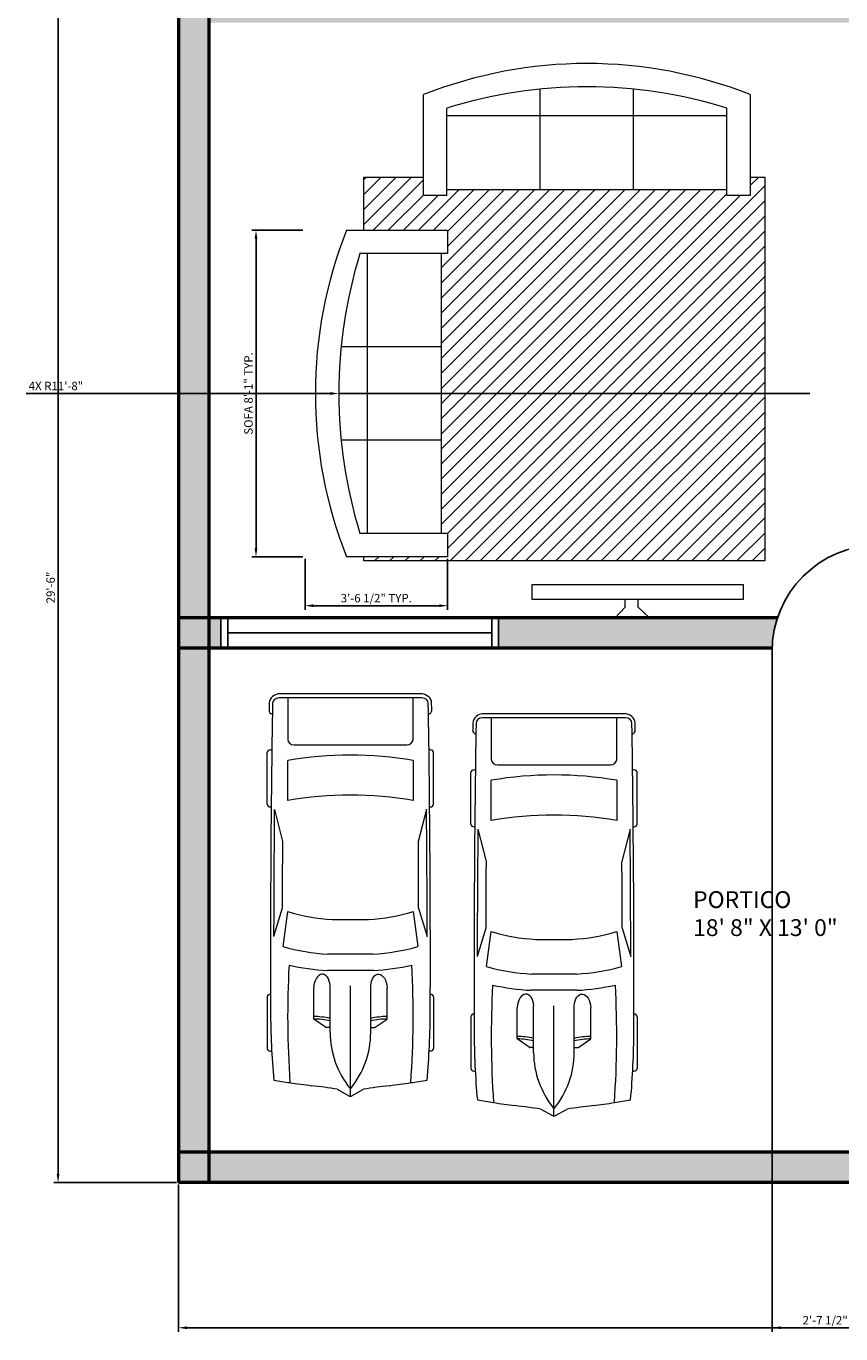
# Model space of a CAD drawing. Units: millimetres. Extents: x 2481 to 3088, y 720 to 1513.
# Tile 1 of 4: x 2481 to 2723, y 720 to 1109. Entities that reach past the tile are written whole.
import ezdxf

# ---------------------------------------------------------------- set-up
doc = ezdxf.new("R2010")
doc.units = ezdxf.units.MM
for name, color, linetype, lineweight in [('A-EQPM', 2, 'Continuous', 18), ('A-SITE-VEHC', 2, 'Continuous', 13), ('A-WALL-PATT', 5, 'Continuous', 13), ('DIMENSIONS', 10, 'Continuous', 18), ('DOORS', 213, 'Continuous', 25), ('FURNITURE', 2, 'Continuous', 18), ('TEXT', 80, 'Continuous', 25), ('WALLS', 150, 'Continuous', 50), ('WINDOWS', 23, 'Continuous', 25)]:
    doc.layers.add(name, color=color, linetype=linetype, lineweight=lineweight)
doc.layers.add('A-FLOR-PATT', color=152, linetype='Continuous', lineweight=13, true_color=0x2776bb)
doc.styles.get("Standard").update_dxf_attribs({"font": 'arial.ttf'})
doc.dimstyles.new('ISO-25', dxfattribs={"dimtxt": 2.5, "dimasz": 2.5, "dimexe": 1.25, "dimexo": 0.625, "dimtad": 1, "dimdec": 0, "dimlunit": 3, "dimtxsty": 'Standard', "dimcen": 2.5, "dimadec": 0, "dimazin": 0, "dimtfac": 1, "dimtdec": 0, "dimtmove": 0, "dimatfit": 3, "dimfxl": 1, "dimarcsym": 0})

# ---------------------------------------------------------------- blocks, each defined once
blk = doc.blocks.new('*U2')
for p, q in [((0, 0), (0, -6)), ((40, 0), (40, -6))]:
    blk.add_line(p, q)
blk.add_lwpolyline([(0, 0), (0, 40), (1.75, 40), (1.75, 0)], close=True)
blk.add_arc((0, 0), 40, 0, 90)
blk = doc.blocks.new('*U4')
for p, q in [((0, 4), (0, 0)), ((36, 4), (36, 0)), ((0, 2), (36, 2))]:
    blk.add_line(p, q)
blk = doc.blocks.new('Sofa - Roundback 7 ft.')
for p, q in [((-12.00002, -32.4421), (-12.00003, -6.5971)), ((11.99997, -32.4421), (11.99998, -6.5971)), ((-36.000027, -34), (-36.000027, -11.4696)), ((-35.999844, -13.3819), (35.9998, -13.3819)), ((35.99998, -34), (35.99998, -11.4696)), ((-36.000027, -32.4421), (35.99998, -32.4421))]:
    blk.add_line(p, q)
for points in [[(-36.000027, -34), (-42.000027, -34), (-42.000027, -8)], [(41.99998, -8), (41.99998, -34), (35.99998, -34)]]:
    blk.add_lwpolyline(points)
for centre, radius, start, end in [((0, -114.25), 114.25, 68.43141, 111.5686), ((-0.00001, -127.1968), 121.1968, 72.72033, 107.2797)]:
    blk.add_arc(centre, radius, start, end)
blk = doc.blocks.new('*U13')
for p, q in [((21.1, 37.41), (21.1, 36.83)), ((46.55, 38.89), (22.35, 38.89)), ((47.8, 37.39), (47.8, 37.41)), ((135.45, 37.07), (135.45, 37.41)), ((136.7, 38.89), (160.9, 38.89)), ((162.15, 37.41), (162.15, 36.77)), ((70.03, 31.54), (86.41, 29.35)), ((87.99, 31.87), (74.76, 35.92)), ((134.31, 35.6), (119.29, 31.78)), ((186.47, -33.5), (186.47, 33.5)), ((188.4, -32.76), (188.4, 32.76)), ((138.42, 29.35), (157.25, 29.35)), ((164.52, 26.39), (164.52, -26.39)), ((186.47, 29.35), (167.01, 29.35)), ((32.27, 11.63), (36.13, 17.17)), ((36.13, 17.17), (50.94, 17.17)), ((3.27, 6.13), (0.1, 0.41)), ((29.77, 9.51), (51.68, 9.51)), ((32.12, 9.51), (32.12, 11.15)), ((58.92, -10.77), (58.92, 10.77)), ((66.55, -10.53), (66.55, 10.53)), ((82.74, 8.5), (82.74, -8.5)), ((186.47, -10.53), (186.47, 10.53)), ((0, 0), (51.68, 0)), ((0.1, -0.41), (3.27, -6.13)), ((29.77, -9.51), (51.68, -9.51)), ((32.12, -9.51), (32.12, -11.15)), ((32.27, -11.63), (36.13, -17.17)), ((36.13, -17.17), (50.94, -17.17)), ((86.41, -29.35), (70.03, -31.54)), ((157.25, -29.35), (138.42, -29.35)), ((167.01, -29.35), (186.47, -29.35)), ((87.99, -31.87), (74.76, -35.92)), ((134.31, -35.6), (119.29, -31.78)), ((21.1, -37.41), (21.1, -36.83)), ((46.55, -38.89), (22.35, -38.89)), ((47.8, -37.39), (47.8, -37.41)), ((135.45, -37.07), (135.45, -37.41)), ((136.7, -38.89), (160.9, -38.89)), ((162.15, -37.41), (162.15, -36.77))]:
    blk.add_line(p, q)
for centre, major_axis, ratio, start_param, end_param in [((41.19, -490.86), (0, 528.23), 0.842304, 0.00281, 0.075598), ((22.35, 37.41), (0, -1.48), 0.842304, 3.141593, 4.712389), ((64.48, -10555.62), (0, 10593.03), 0.842304, -0.013397, 0.002797), ((46.55, 37.41), (0, 1.48), 0.842304, -1.570796, 0), ((136.7, 37.41), (0, -1.48), 0.842304, 3.141593, 4.712389), ((160.9, 37.41), (0, 1.48), 0.842304, -1.570796, 0), ((180.63, 35.84), (0, 2.22), 0.842304, -0.013017, 1.249894), ((64.48, -10556.36), (0, 10595.31), 0.842304, -0.013397, -0.013017), ((183.98, 32.76), (0, -5.25), 0.842304, 1.570796, 3.128196), ((266.03, -27.52), (0, 313.31), 0.842304, 1.367076, 1.39176), ((135.29, 5.39), (0, 81.77), 0.842304, 1.245306, 1.50788), ((64.48, -10555.62), (0, -10591.55), 0.842304, 3.133765, 3.140441), ((95.79, -3666.35), (0, -3698.24), 0.842304, 3.134049, 3.144098), ((183.98, 33.5), (0, -2.96), 0.842304, 1.570796, 3.128196), ((259.18, -27.52), (0, -305.3), 0.842304, 4.528606, 4.561838), ((37.47, -593.96), (0, -623.33), 0.842304, 3.096046, 3.200911), ((134.4, 5.39), (0, -89.78), 0.842304, 4.449482, 4.652344), ((149.6, 2.8), (0, -79.58), 0.842304, 4.372215, 4.640744), ((17.08, 0), (0, 147.02), 0.842304, 4.511394, 4.913384), ((35.91, 0), (0, 147.02), 0.842304, 4.511394, 4.913384), ((167.01, 26.39), (0, 2.96), 0.842304, 0, 1.570796), ((-204.49, 52.4), (0, -250.96), 0.842304, 1.385369, 1.434372), ((13.04, 17.01), (0, 27.42), 0.842304, 4.435146, 4.718221), ((14.2, 17.01), (0, 27.42), 0.842304, 4.435146, 4.718221), ((50.79, 13.34), (6.34, -0.36), 0.603834, -1.395552, 1.581315), ((29.77, -46.66), (0, 56.17), 0.842304, 0, 0.590319), ((32.75, 11.15), (0, 0.74), 0.842304, 0.879714, 1.570796), ((0.62, 0), (0, -0.74), 0.842304, 4.131459, 5.293319), ((29.77, 46.66), (0, 56.17), 0.842304, 2.551274, 3.141593), ((-204.49, -52.4), (0, 250.96), 0.842304, -1.434372, -1.385369), ((32.75, -11.15), (0, -0.74), 0.842304, 4.712389, 5.403472), ((13.04, -17.01), (0, -27.42), 0.842304, 1.564964, 1.848039), ((14.2, -17.01), (0, -27.42), 0.842304, 1.564964, 1.848039), ((134.4, -5.39), (0, -89.78), 0.842304, -1.510751, -1.307889), ((135.29, -5.39), (0, -81.77), 0.842304, -1.50788, -1.245306), ((149.6, -2.8), (0, -79.58), 0.842304, -1.499151, -1.230623), ((259.18, 27.52), (0, 305.3), 0.842304, 1.721348, 1.754579), ((266.03, 27.52), (0, 313.31), 0.842304, 1.749832, 1.774517), ((37.47, 593.96), (0, -623.33), 0.842304, -0.059319, 0.045547), ((167.01, -26.39), (0, -2.96), 0.842304, 4.712389, 6.283185), ((41.19, 490.86), (0, -528.23), 0.842304, -0.075598, -0.00281), ((64.48, 10555.62), (0, 10593.03), 0.842304, 3.138796, 3.15499), ((64.48, 10555.62), (0, -10591.55), 0.842304, 0.001152, 0.007828), ((95.79, 3666.35), (0, -3698.24), 0.842304, -0.002505, 0.007544), ((180.63, -35.84), (0, -2.22), 0.842304, -1.249894, 0.013017), ((183.98, -33.5), (0, 2.96), 0.842304, 3.15499, 4.712389), ((183.98, -32.76), (0, -5.25), 0.842304, 0.013397, 1.570796), ((22.35, -37.41), (0, 1.48), 0.842304, 1.570796, 3.141593), ((46.55, -37.41), (0, -1.48), 0.842304, 0, 1.570796), ((136.7, -37.41), (0, -1.48), 0.842304, -1.570796, 0), ((160.9, -37.41), (0, 1.48), 0.842304, 3.141593, 4.712389), ((64.48, 10556.36), (0, 10595.31), 0.842304, 3.15461, 3.15499)]:
    blk.add_ellipse(centre, major_axis=major_axis, ratio=ratio, start_param=start_param, end_param=end_param)
at = {"extrusion": (0, 0, -1)}
blk.add_ellipse((50.79, -13.34), major_axis=(6.34, 0.36), ratio=0.603834, start_param=-1.395552, end_param=1.581315, dxfattribs=at)
blk = doc.blocks.new('*D27')
at = {"layer": 'Defpoints', "color": 0, "transparency": 16777216}
for p in [(2549.54, 1048.77), (2564.11, 1048.77), (2564.11, 951.65)]:
    blk.add_point(p, dxfattribs=at)
at = {"layer": 'DIMENSIONS', "color": 0, "lineweight": -2, "transparency": 16777216}
for p, q in [((2563.48, 1048.77), (2548.29, 1048.77)), ((2549.54, 954.15), (2549.54, 1046.27)), ((2563.48, 951.65), (2548.29, 951.65))]:
    blk.add_line(p, q, dxfattribs=at)
at = {"layer": 'DIMENSIONS', "color": 0, "transparency": 16777216}
for points in [[(2549.12, 1046.27), (2549.95, 1046.27), (2549.54, 1048.77)], [(2549.12, 954.15), (2549.95, 954.15), (2549.54, 951.65)]]:
    blk.add_solid(points, dxfattribs=at)
at = {"layer": 'DIMENSIONS', "color": 0, "transparency": 16777216, "insert": (2547.62, 1000.21), "char_height": 2.5, "attachment_point": 5, "rotation": 90}
blk.add_mtext('SOFA 8\'-1" TYP.', dxfattribs=at)
blk = doc.blocks.new('*D28')
at = {"layer": 'Defpoints', "color": 0, "transparency": 16777216}
for p in [(2564.11, 951.65), (2606.5, 951.65), (2564.11, 937.09)]:
    blk.add_point(p, dxfattribs=at)
at = {"layer": 'DIMENSIONS', "color": 0, "lineweight": -2, "transparency": 16777216}
for p, q in [((2564.11, 951.03), (2564.11, 935.84)), ((2606.5, 951.03), (2606.5, 935.84)), ((2604, 937.09), (2566.61, 937.09))]:
    blk.add_line(p, q, dxfattribs=at)
at = {"layer": 'DIMENSIONS', "color": 0, "transparency": 16777216}
for points in [[(2566.61, 937.5), (2566.61, 936.67), (2564.11, 937.09)], [(2604, 937.5), (2604, 936.67), (2606.5, 937.09)]]:
    blk.add_solid(points, dxfattribs=at)
at = {"layer": 'DIMENSIONS', "color": 0, "transparency": 16777216, "insert": (2585.3, 939), "char_height": 2.5, "attachment_point": 5}
blk.add_mtext('3\'-6 1/2" TYP.', dxfattribs=at)
blk = doc.blocks.new('*D37')
at = {"layer": 'Defpoints', "color": 0, "transparency": 16777216}
for p in [(2526.5, 765.49), (3046.5, 765.49), (3046.5, 722.28)]:
    blk.add_point(p, dxfattribs=at)
at = {"layer": 'DIMENSIONS', "color": 0, "lineweight": -2, "transparency": 16777216}
for p, q in [((2526.5, 764.86), (2526.5, 721.03)), ((3046.5, 764.86), (3046.5, 721.03)), ((2529, 722.28), (3044, 722.28))]:
    blk.add_line(p, q, dxfattribs=at)
at = {"layer": 'DIMENSIONS', "color": 0, "transparency": 16777216}
for points in [[(2529, 722.7), (2529, 721.86), (2526.5, 722.28)], [(3044, 722.7), (3044, 721.86), (3046.5, 722.28)]]:
    blk.add_solid(points, dxfattribs=at)
at = {"layer": 'DIMENSIONS', "color": 0, "transparency": 16777216, "insert": (2786.5, 724.18), "char_height": 2.5, "attachment_point": 5}
blk.add_mtext('43\'-4"', dxfattribs=at)
blk = doc.blocks.new('*D40')
at = {"layer": 'Defpoints', "color": 0, "transparency": 16777216}
for p in [(2490.69, 1119.49), (2526.5, 1119.49), (2526.5, 765.49)]:
    blk.add_point(p, dxfattribs=at)
at = {"layer": 'DIMENSIONS', "color": 0, "lineweight": -2, "transparency": 16777216}
for p, q in [((2525.87, 1119.49), (2489.44, 1119.49)), ((2490.69, 767.99), (2490.69, 1116.99)), ((2525.87, 765.49), (2489.44, 765.49))]:
    blk.add_line(p, q, dxfattribs=at)
at = {"layer": 'DIMENSIONS', "color": 0, "transparency": 16777216}
for points in [[(2490.28, 1116.99), (2491.11, 1116.99), (2490.69, 1119.49)], [(2490.28, 767.99), (2491.11, 767.99), (2490.69, 765.49)]]:
    blk.add_solid(points, dxfattribs=at)
at = {"layer": 'DIMENSIONS', "color": 0, "transparency": 16777216, "insert": (2488.79, 942.49), "char_height": 2.5, "attachment_point": 5, "rotation": 90}
blk.add_mtext('29\'-6"', dxfattribs=at)
blk = doc.blocks.new('*D45')
at = {"layer": 'Defpoints', "color": 0, "transparency": 16777216}
for p in [(2703, 924.49), (2734.57, 924.49), (2734.57, 722.28)]:
    blk.add_point(p, dxfattribs=at)
at = {"layer": 'DIMENSIONS', "color": 0, "lineweight": -2, "transparency": 16777216}
for p, q in [((2703, 923.86), (2703, 721.03)), ((2734.57, 923.86), (2734.57, 721.03)), ((2705.5, 722.28), (2732.07, 722.28))]:
    blk.add_line(p, q, dxfattribs=at)
at = {"layer": 'DIMENSIONS', "color": 0, "transparency": 16777216}
for points in [[(2705.5, 722.7), (2705.5, 721.86), (2703, 722.28)], [(2732.07, 722.7), (2732.07, 721.86), (2734.57, 722.28)]]:
    blk.add_solid(points, dxfattribs=at)
at = {"layer": 'DIMENSIONS', "color": 0, "transparency": 16777216, "insert": (2718.78, 724.2), "char_height": 2.5, "attachment_point": 5}
blk.add_mtext('2\'-7 1/2"', dxfattribs=at)
blk = doc.blocks.new('*D47')
at = {"layer": 'Defpoints', "color": 0, "transparency": 16777216}
for p in [(2574.13, 1000.21), (2714.25, 1000.21)]:
    blk.add_point(p, dxfattribs=at)
at = {"layer": 'DIMENSIONS', "color": 0, "lineweight": -2, "transparency": 16777216}
for p, q in [((2481.2, 1000.21), (2571.63, 1000.21)), ((2714.25, 1000.21), (2574.13, 1000.21))]:
    blk.add_line(p, q, dxfattribs=at)
at = {"layer": 'DIMENSIONS', "color": 0, "transparency": 16777216}
blk.add_solid([(2571.63, 1000.63), (2571.63, 999.8), (2574.13, 1000.21)], dxfattribs=at)
at = {"layer": 'DIMENSIONS', "color": 0, "transparency": 16777216, "insert": (2490.05, 1002.12), "char_height": 2.5, "attachment_point": 5, "rotation": 359.9998}
blk.add_mtext('4X R11\'-8"', dxfattribs=at)

msp = doc.modelspace()

# ---------------------------------------------------------------- hatches: boundary and pattern name
at = {"layer": 'A-FLOR-PATT'}
h = msp.add_hatch(dxfattribs=at)
h.set_pattern_fill('ANSI31', color=256)
h.paths.add_polyline_path([(2700.86, 1064.61), (2696.49, 1064.61), (2696.49, 1059.06), (2689.56, 1059.06), (2689.56, 1060.86), (2606.31, 1060.86), (2606.31, 1059.06), (2599.37, 1059.06), (2599.37, 1064.61), (2581.59, 1064.61), (2581.59, 1048.77), (2606.5, 1048.77), (2606.5, 1041.84), (2604.7, 1041.84), (2604.7, 958.59), (2606.5, 958.59), (2606.5, 951.65), (2581.59, 951.65), (2581.59, 950.38), (2700.86, 950.38)])
at = {"layer": 'A-WALL-PATT'}
h = msp.add_hatch(color=256, dxfattribs=at)
h.dxf.hatch_style = 1
h.paths.add_polyline_path([(2599.5, 1473.49), (2590.5, 1473.49), (2590.5, 1464.49), (2599.5, 1464.49)])
h.paths.add_polyline_path([(2599.5, 1464.49), (2590.5, 1464.49), (2590.5, 1447.8), (2599.5, 1447.8)])
h.paths.add_polyline_path([(2625.38, 1473.49), (2599.5, 1473.49), (2599.5, 1464.49), (2625.38, 1464.49)])
h.paths.add_polyline_path([(2805.36, 1473.49), (2710.95, 1473.49), (2710.95, 1464.49), (2805.36, 1464.49)])
h.paths.add_polyline_path([(2922.5, 1473.49), (2830.18, 1473.49), (2830.18, 1464.49), (2922.5, 1464.49)])
h.paths.add_polyline_path([(2931.5, 1473.49), (2922.5, 1473.49), (2922.5, 1464.49), (2931.5, 1464.49)])
h.paths.add_polyline_path([(2931.5, 1464.49), (2922.5, 1464.49), (2922.5, 1402.56), (2926.01, 1402.56, -0.043673), (2931.5, 1402.08)])
h.paths.add_polyline_path([(2931.5, 1368.49), (2922.5, 1368.49), (2922.5, 1359.49), (2931.5, 1359.49)])
h.paths.add_polyline_path([(2922.5, 1296.49), (2675.15, 1296.49), (2675.15, 1287.49), (2922.5, 1287.49)])
h.paths.add_polyline_path([(2931.5, 1294.49), (2922.5, 1294.49), (2922.5, 1287.49), (2922.5, 1285.49), (2931.5, 1285.49)])
h.paths.add_polyline_path([(3037.5, 1294.49), (2931.5, 1294.49), (2931.5, 1285.49), (3037.5, 1285.49)])
h.paths.add_polyline_path([(3046.5, 1294.49), (3037.5, 1294.49), (3037.5, 1285.49), (3046.5, 1285.49)])
h.paths.add_polyline_path([(3046.5, 1316.66), (3037.5, 1316.66), (3037.5, 1294.49), (3046.5, 1294.49)])
h.paths.add_polyline_path([(3046.5, 1359.49), (3037.5, 1359.49), (3037.5, 1343.26), (3046.5, 1343.26)])
h.paths.add_polyline_path([(3046.5, 1368.49), (3037.5, 1368.49), (3037.5, 1359.49), (3046.5, 1359.49)])
h.paths.add_polyline_path([(3037.5, 1368.49), (2931.5, 1368.49), (2931.5, 1359.49), (3037.5, 1359.49)])
h.paths.add_polyline_path([(2599.5, 1361.25), (2590.5, 1361.25), (2590.5, 1233.6), (2599.5, 1233.6)])
h.paths.add_polyline_path([(2535.5, 1110.49), (2526.5, 1110.49), (2526.5, 933.49), (2535.5, 933.49)])
h.paths.add_polyline_path([(2535.5, 1119.49), (2526.5, 1119.49), (2526.5, 1110.49), (2535.5, 1110.49)])
h.paths.add_polyline_path([(2590.5, 1119.49), (2535.5, 1119.49), (2535.5, 1110.49), (2590.5, 1110.49)])
h.paths.add_polyline_path([(2599.5, 1119.49), (2594.5, 1119.49), (2590.5, 1119.49), (2590.5, 1110.49), (2594.5, 1110.49), (2599.5, 1110.49)])
h.paths.add_polyline_path([(2599.5, 1148.41), (2590.5, 1148.41), (2590.5, 1119.49), (2594.5, 1119.49), (2599.5, 1119.49)])
h.paths.add_polyline_path([(2770.14, 1119.49), (2599.5, 1119.49), (2599.5, 1110.49), (2770.14, 1110.49)])
h.paths.add_polyline_path([(3037.5, 1473.49), (2931.5, 1473.49), (2931.5, 1464.49), (3037.5, 1464.49)])
h.paths.add_polyline_path([(3046.5, 1473.49), (3037.5, 1473.49), (3037.5, 1464.49), (3046.5, 1464.49)])
h.paths.add_polyline_path([(2535.5, 842.83), (2535.5, 924.49), (2526.5, 924.49), (2526.5, 774.49), (2535.5, 774.49)])
h.paths.add_polyline_path([(2535.5, 774.49), (2526.5, 774.49), (2526.5, 765.49), (2535.5, 765.49)])
h.paths.add_polyline_path([(3037.5, 774.49), (2945.5, 774.49), (2852.34, 774.49), (2852.34, 765.49), (3037.5, 765.49)])
h.paths.add_polyline_path([(3046.5, 774.49), (3037.5, 774.49), (3037.5, 765.49), (3046.5, 765.49)])
h.paths.add_polyline_path([(3046.5, 882.49), (3037.5, 882.49), (3037.5, 774.49), (3046.5, 774.49)])
h.paths.add_polyline_path([(2768.5, 774.49), (2759.5, 774.49), (2759.5, 765.49), (2768.5, 765.49)])
h.paths.add_polyline_path([(2759.5, 774.49), (2535.5, 774.49), (2535.5, 765.49), (2759.5, 765.49)])
h.paths.add_polyline_path([(2768.5, 781.94), (2759.5, 781.94), (2759.5, 774.49), (2768.5, 774.49)])
h.paths.add_polyline_path([(2768.5, 1015.49), (2759.5, 1015.49), (2759.5, 933.49), (2768.5, 933.49)])
h.paths.add_polyline_path([(2768.5, 933.49), (2759.5, 933.49), (2759.5, 924.49), (2768.5, 924.49)])
h.paths.add_polyline_path([(2768.5, 924.49), (2759.5, 924.49), (2759.5, 864.16), (2768.5, 864.16)])
h.paths.add_polyline_path([(2759.5, 933.49), (2734.57, 933.49), (2734.57, 924.49), (2759.5, 924.49)])
h.paths.add_polyline_path([(2954.5, 1015.49), (2945.5, 1015.49), (2945.5, 842.83), (2954.5, 842.83)])
h.paths.add_polyline_path([(2954.5, 1024.49), (2945.5, 1024.49), (2945.5, 1015.49), (2954.5, 1015.49)])
h.paths.add_polyline_path([(2945.5, 1024.49), (2808.62, 1024.49), (2808.62, 1022.52, -0.056199), (2807.82, 1015.49), (2945.5, 1015.49)])
h.paths.add_polyline_path([(3037.5, 1024.49), (2954.5, 1024.49), (2954.5, 1015.49), (3037.5, 1015.49)])
h.paths.add_polyline_path([(3046.5, 1024.49), (3037.5, 1024.49), (3037.5, 1015.49), (3046.5, 1015.49)])
h.paths.add_polyline_path([(3046.5, 1015.49), (3037.5, 1015.49), (3037.5, 994.13), (3046.5, 994.13)])
h.paths.add_polyline_path([(3046.5, 928.1), (3037.5, 928.1), (3037.5, 891.49), (3046.5, 891.49)])
h.paths.add_polyline_path([(3046.5, 891.49), (3037.5, 891.49), (3037.5, 882.49), (3046.5, 882.49)])
h.paths.add_polyline_path([(3037.5, 891.49), (2987.62, 891.49), (2987.62, 882.49), (3037.5, 882.49)])
h.paths.add_polyline_path([(2768.5, 1024.49), (2759.5, 1024.49), (2759.5, 1015.49), (2768.5, 1015.49)])
h.paths.add_polyline_path([(2777.03, 1022.52), (2777.03, 1024.49), (2768.5, 1024.49), (2768.5, 1015.49), (2777.03, 1015.49)])
h = msp.add_hatch(color=256, dxfattribs=at)
h.dxf.hatch_style = 1
h.paths.add_polyline_path([(2535.5, 933.49), (2526.5, 933.49), (2526.5, 924.49), (2535.5, 924.49)])
h.paths.add_polyline_path([(2539.07, 933.49), (2535.5, 933.49), (2535.5, 924.49), (2539.07, 924.49)])
h.paths.add_polyline_path([(2704.6, 933.49), (2621.64, 933.49), (2621.64, 924.49), (2703, 924.49, -0.072743)])

# ---------------------------------------------------------------- linework, layer by layer
at = {"layer": 'A-EQPM'}
for p, q in [((2659.2, 938.95), (2659.2, 936.54)), ((2663.04, 938.95), (2663.04, 936.7)), ((2659.2, 936.54), (2656.35, 933.49)), ((2663.04, 936.7), (2666.52, 933.49))]:
    msp.add_line(p, q, dxfattribs=at)
msp.add_lwpolyline([(2631.65, 943.41), (2694.42, 943.41), (2694.42, 938.95), (2631.65, 938.95)], close=True, dxfattribs=at)
at = {"layer": 'FURNITURE'}
for p, q in [((2581.59, 1064.61), (2599.37, 1064.61)), ((2581.59, 1048.77), (2581.59, 1064.61)), ((2696.49, 1064.61), (2700.86, 1064.61)), ((2700.86, 1064.61), (2700.86, 950.38)), ((2581.59, 950.38), (2581.59, 951.65)), ((2700.86, 950.38), (2581.59, 950.38))]:
    msp.add_line(p, q, dxfattribs=at)
at = {"layer": 'WALLS'}
for p, q in [((2526.5, 1119.49), (2526.5, 765.49)), ((2535.5, 1119.49), (2535.5, 774.49)), ((2704.6, 933.49), (2526.5, 933.49)), ((2703, 924.49), (2526.5, 924.49)), ((2535.5, 842.83), (2535.5, 765.49)), ((2839.77, 774.49), (2526.5, 774.49)), ((2839.77, 765.49), (2526.5, 765.49))]:
    msp.add_line(p, q, dxfattribs=at)
at = {"layer": 'WINDOWS'}
for p, q in [((2539.07, 933.49), (2539.07, 924.49)), ((2621.64, 933.49), (2621.64, 924.49))]:
    msp.add_line(p, q, dxfattribs=at)

# ---------------------------------------------------------------- block references
at = {"layer": 'A-SITE-VEHC', "xscale": 0.6353957798837438, "yscale": 0.6353957798837438, "zscale": 0.6353957798837438, "rotation": 90}
for p in [(2577.61, 791.16), (2638.14, 785.23)]:
    msp.add_blockref('*U13', p, dxfattribs=at)
at = {"layer": 'DOORS', "xscale": -0.7896024204950681, "yscale": 0.7896024204950681, "zscale": 0.7896024204950681, "rotation": 359.9999960046612}
msp.add_blockref('*U2', (2734.57, 923.5), dxfattribs=at)
at = {"layer": 'FURNITURE', "xscale": 1.15619311164389, "yscale": 1.15619311164389, "zscale": 1.15619311164389}
msp.add_blockref('Sofa - Roundback 7 ft.', (2647.93, 1098.37), dxfattribs=at)
at = {"layer": 'FURNITURE', "xscale": 1.15619311164389, "yscale": 1.15619311164389, "zscale": 1.15619311164389, "rotation": 89.99999999999999}
msp.add_blockref('Sofa - Roundback 7 ft.', (2567.19, 1000.21), dxfattribs=at)
at = {"layer": 'WINDOWS', "xscale": 2.179725659021641, "yscale": 2.179725659021641, "zscale": 2.179725659021641}
msp.add_blockref('*U4', (2541.17, 924.65), dxfattribs=at)

# ---------------------------------------------------------------- texts
at = {"layer": 'TEXT', "insert": (2679.5, 852.15), "char_height": 5, "attachment_point": 1}
msp.add_mtext_dynamic_manual_height_columns('PORTICO\\P18\' 8" X 13\' 0"', width=48.9564, gutter_width=12.5, heights=[0], dxfattribs=at)

# ---------------------------------------------------------------- dimensions: what is measured, and where the dimension line sits
at = {"layer": 'DIMENSIONS'}
dim = msp.add_linear_dim(base=(2490.69, 1119.49), p1=(2526.5, 765.49), p2=(2526.5, 1119.49), angle=90, dimstyle='ISO-25', override={"dimdec": 1, "dimlfac": 1, "dimrnd": 0, "dimzin": 1, "dimdsep": 46, "dimlunit": 4, "dimfrac": 2}, dxfattribs=at)
dim.commit()
dim.dimension.update_dxf_attribs({"geometry": '*D40', "text_midpoint": (2488.79, 942.49)})
for base, p1, p2, angle, text, picture, middle in [((2549.54, 1048.77), (2564.11, 951.65), (2564.11, 1048.77), 90, 'SOFA <> TYP.', '*D27', (2547.62, 1000.21)), ((2564.11, 937.09), (2606.5, 951.65), (2564.11, 951.65), 180, '<> TYP.', '*D28', (2585.3, 939))]:
    dim = msp.add_linear_dim(base=base, p1=p1, p2=p2, angle=angle, text=text, dimstyle='ISO-25', override={"dimdec": 1, "dimlfac": 1, "dimrnd": 0, "dimzin": 1, "dimdsep": 46, "dimlunit": 4, "dimfrac": 2}, dxfattribs=at)
    dim.commit()
    dim.dimension.update_dxf_attribs({"geometry": picture, "text_midpoint": middle})
dim = msp.add_radius_dim(center=(2714.25, 1000.21), mpoint=(2574.13, 1000.21), text='4X <>', dimstyle='ISO-25', override={"dimdec": 1, "dimlfac": 1, "dimrnd": 0, "dimzin": 1, "dimdsep": 46, "dimlunit": 4, "dimfrac": 2}, dxfattribs=at)
dim.commit()
dim.dimension.update_dxf_attribs({"geometry": '*D47', "text_midpoint": (2490.05, 1000.21), "dimtype": 164})
for base, p1, p2, picture, middle in [((2734.57, 722.28), (2703, 924.49), (2734.57, 924.49), '*D45', (2718.78, 724.2)), ((3046.5, 722.28), (2526.5, 765.49), (3046.5, 765.49), '*D37', (2786.5, 724.18))]:
    dim = msp.add_linear_dim(base=base, p1=p1, p2=p2, dimstyle='ISO-25', override={"dimdec": 1, "dimlfac": 1, "dimrnd": 0, "dimzin": 1, "dimdsep": 46, "dimlunit": 4, "dimfrac": 2}, dxfattribs=at)
    dim.commit()
    dim.dimension.update_dxf_attribs({"geometry": picture, "text_midpoint": middle})

doc.saveas('drawing.dxf')
